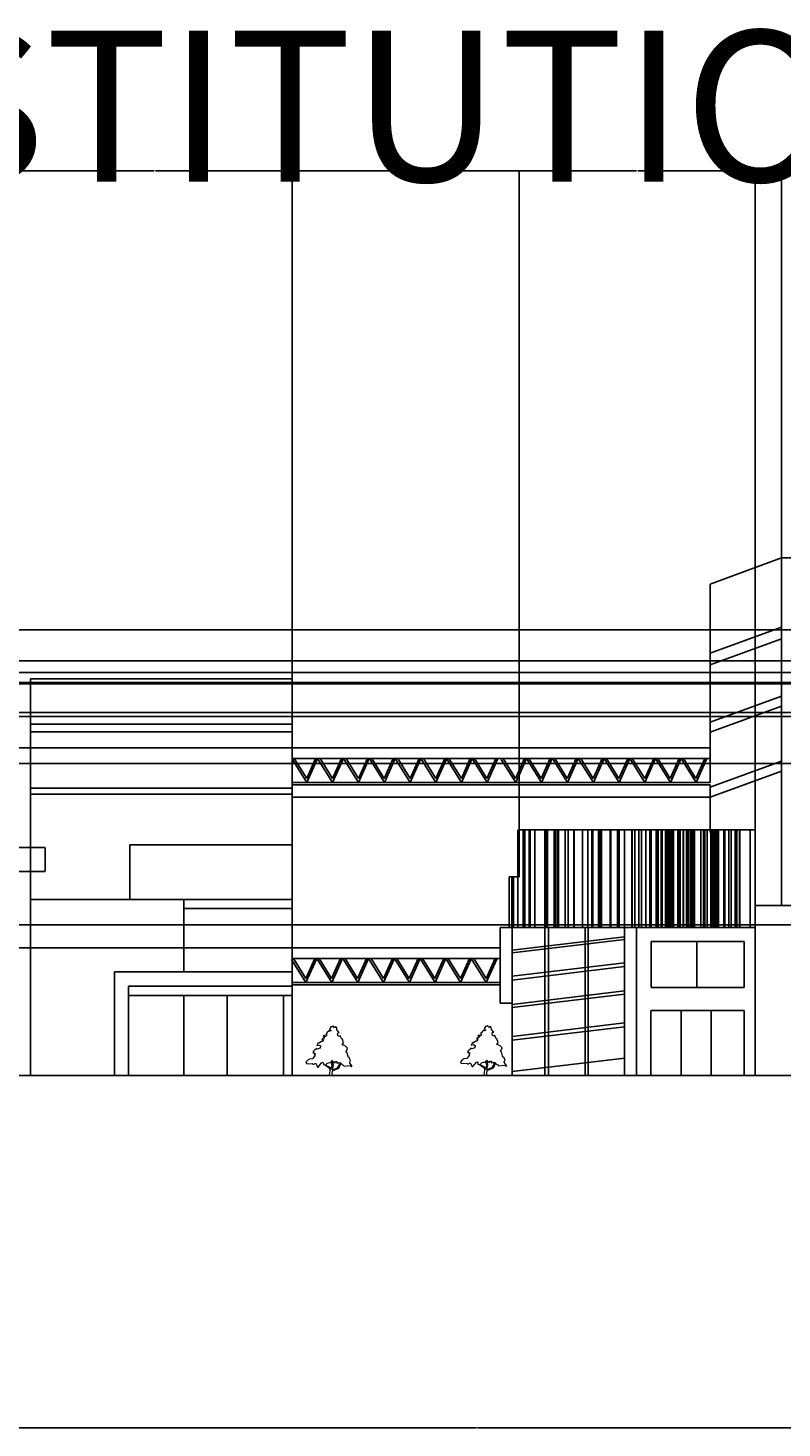
# Model space of a CAD drawing. Units: inches. Extents: x -2248 to 2617, y -128 to 922.
# Tile 4 of 7: x -152 to 413, y -128 to 922. Entities that reach past the tile are written whole.
import ezdxf

# ---------------------------------------------------------------- set-up
doc = ezdxf.new("R2010")
doc.units = ezdxf.units.IN
doc.header["$MEASUREMENT"] = 0
for name, color, linetype, lineweight in [('A-ANNO-DIMS', 2, 'Continuous', 18), ('A-ANNO-TEXT', 7, 'Continuous', 25), ('A-ELEV', 7, 'Continuous', 25), ('L-PLNT', 3, 'Continuous', 18)]:
    doc.layers.add(name, color=color, linetype=linetype, lineweight=lineweight)
doc.styles.get("Standard").update_dxf_attribs({"font": 'arial.ttf'})
doc.dimstyles.get("Standard").update_dxf_attribs({"dimtxt": 0.18, "dimasz": 0.18, "dimexe": 0.18, "dimexo": 0.0625, "dimgap": 0.09, "dimtad": 0, "dimtih": 1, "dimtoh": 1, "dimdec": 4, "dimzin": 0, "dimdsep": 46, "dimtxsty": 'Standard', "dimcen": 0.09, "dimadec": 0, "dimazin": 0, "dimtfac": 1, "dimtdec": 4, "dimtofl": 0, "dimtmove": 0, "dimatfit": 3, "dimfxl": 1, "dimtolj": 1, "dimtzin": 0, "dimarcsym": 0})

# ---------------------------------------------------------------- blocks, each defined once
blk = doc.blocks.new('*U2')
for points in [[(22.0124, 137.721), (18.5475, 141.5624), (15.5282, 138.2446), (13.8028, 139.3505), (13.3714, 142.1153), (11.2148, 143.2214), (8.1954, 140.4564), (4.7447, 141.0094), (2.1567, 136.0326), (2.1567, 131.6088), (5.6074, 129.9499), (3.0193, 128.2909), (0.4313, 130.5029), (-6.9015, 123.3141), (-6.9015, 121.6552), (-9.9208, 119.9963), (-9.0581, 118.3373), (-6.9015, 115.0195), (-10.7835, 112.2546), (-14.6656, 115.0195), (-16.8222, 114.4665), (-17.6849, 112.2546), (-14.6656, 111.7016), (-14.2342, 107.2778), (-17.6065, 107.8307), (-21.5669, 103.9599), (-17.2536, 103.4069), (-18.9789, 97.8771), (-22.8609, 97.3241), (-27.1743, 94.5593), (-32.3504, 91.7944), (-32.7817, 94.0063), (-36.6638, 85.7116), (-29.7624, 87.3705), (-25.449, 84.6056), (-26.743, 77.9699), (-34.507, 75.205), (-37.9578, 77.4169), (-39.2518, 74.099), (-42.2711, 73.5461), (-44.8592, 70.2282), (-47.8786, 66.3574), (-43.9965, 63.0395), (-41.4085, 64.6985), (-44.3346, 59.8898), (-42.2089, 60.1377), (-42.5159, 55.7849), (-49.6039, 46.4502), (-58.2307, 45.8972), (-62.1127, 43.6853), (-68.5828, 36.4966), (-65.9947, 32.0727), (-50.0352, 32.6257), (-47.0159, 30.4138), (-39.6831, 33.7317), (-34.507, 22.6721), (-32.3504, 22.6721), (-22.4296, 34.8376), (-19.4102, 36.4966), (-17.2536, 33.7317), (-17.2536, 29.8608), (-13.8028, 28.7549), (-9.0581, 28.7549), (-7.3328, 32.6257), (-1.7254, 35.3906), (3.8821, 35.9436), (6.4701, 38.1555), (6.9014, 38.7085), (8.1954, 41.4734), (9.9208, 40.3674), (11.2148, 35.9436), (14.2341, 37.6025), (15.0968, 36.4966), (15.9595, 33.7317), (18.9789, 38.7085), (21.9982, 38.7085), (23.2922, 36.4966), (21.9982, 34.2847), (25.4489, 35.3906), (26.743, 33.7317), (29.7623, 35.9436), (32.7817, 34.8376), (38.8204, 28.7549), (41.4084, 27.6489), (43.5651, 25.437), (61.6813, 27.0959), (65.132, 23.7781), (67.7201, 24.884), (60.8186, 33.7317), (60.3873, 37.0495), (62.544, 40.3674), (58.662, 50.874), (56.5053, 50.874), (52.1919, 66.3574), (47.8785, 66.9103), (50.4665, 69.1222), (53.9172, 77.9699), (47.0158, 85.1586), (38.3891, 87.9235), (42.2711, 94.0063)], [(42.2711, 94.0063), (38.8204, 104.5129), (36.6637, 104.5129), (32.3503, 113.9135), (29.7623, 113.3605), (26.743, 113.3605), (24.5862, 117.7844), (25.8802, 123.8671), (29.331, 123.8671), (22.8609, 131.6088), (21.9982, 137.6916)], [(-12.9401, 28.7549), (-2.588, 22.1191), (0.8626, 17.6953), (1.7253, 11.6125), (0, 0)], [(-9.9208, 28.2019), (0, 23.2251), (3.4507, 19.9072), (4.7447, 15.4834), (8.6267, 27.0959), (6.4701, 37.6025)], [(34.5071, 33.1787), (27.1743, 18.2483), (9.0581, 10.5066), (7.7641, 3.8708), (8.1954, 0)], [(8.1954, 40.3674), (11.2148, 27.6489), (8.1954, 13.8245), (24.5862, 19.9072), (32.7817, 34.2847)]]:
    blk.add_lwpolyline(points)
blk = doc.blocks.new('TRUSS-BRIDGE-SEG')
for p, q in [((0, 17.2), (10.8, 0)), ((10.8, 0), (18.9, 17.9)), ((18.8, 17.9), (30.1, 0)), ((30.1, 0), (38.2, 17.9)), ((38.3, 17.9), (49.5, 0)), ((49.5, 0), (57.6, 17.9)), ((57.7, 17.9), (69, 0)), ((69, 0), (77.1, 17.9)), ((77, 17.9), (88.2, 0)), ((88.2, 0), (96.3, 17.9)), ((96.3, 17.9), (107.5, 0)), ((107.5, 0), (115.6, 17.9)), ((115.5, 17.9), (126.7, 0)), ((126.7, 0), (134.8, 17.9)), ((134.7, 17.9), (145.9, 0)), ((145.9, 0), (154, 17.9))]:
    blk.add_line(p, q)
blk = doc.blocks.new('*D15')
at = {"layer": 'A-ANNO-DIMS', "color": 0, "lineweight": -2, "transparency": 16777216}
for p, q in [((-162.3, 307.2), (-139.1, 307.2)), ((-139.3, 307), (-139.3, 298.4)), ((-139.3, 289.5), (-139.3, 298.1)), ((-162.3, 289.3), (-139.1, 289.3))]:
    blk.add_line(p, q, dxfattribs=at)
at = {"layer": 'A-ANNO-DIMS', "color": 0, "transparency": 16777216}
for points in [[(-139.3, 307), (-139.2, 307), (-139.3, 307.2)], [(-139.3, 289.5), (-139.2, 289.5), (-139.3, 289.3)]]:
    blk.add_solid(points, dxfattribs=at)
at = {"layer": 'Defpoints', "color": 0, "transparency": 16777216}
for p in [(-162.4, 307.2), (-139.3, 307.2), (-162.4, 289.3)]:
    blk.add_point(p, dxfattribs=at)
at = {"layer": 'A-ANNO-DIMS', "color": 0, "transparency": 16777216, "insert": (-139.3, 298.2), "char_height": 0.18, "attachment_point": 5}
blk.add_mtext('\\A1;18 TYP.', dxfattribs=at)
blk = doc.blocks.new('*D16')
at = {"layer": 'A-ANNO-DIMS', "color": 0, "lineweight": -2, "transparency": 16777216}
for p, q in [((45.9, 438.4), (2616.5, 438.4)), ((2616.3, 438.3), (2616.3, 287.6)), ((2616.3, 136.6), (2616.3, 287.3)), ((45.9, 136.5), (2616.5, 136.5))]:
    blk.add_line(p, q, dxfattribs=at)
at = {"layer": 'A-ANNO-DIMS', "color": 0, "transparency": 16777216}
for points in [[(2616.2, 438.3), (2616.3, 438.3), (2616.3, 438.4)], [(2616.2, 136.6), (2616.3, 136.6), (2616.3, 136.5)]]:
    blk.add_solid(points, dxfattribs=at)
at = {"layer": 'Defpoints', "color": 0, "transparency": 16777216}
for p in [(45.8, 438.4), (45.8, 136.5), (2616.3, 136.5)]:
    blk.add_point(p, dxfattribs=at)
at = {"layer": 'A-ANNO-DIMS', "color": 0, "transparency": 16777216, "insert": (2616.3, 287.4), "char_height": 0.18, "attachment_point": 5}
blk.add_mtext('\\A1;302', dxfattribs=at)
blk = doc.blocks.new('*D20')
at = {"layer": 'A-ANNO-DIMS', "color": 0, "lineweight": -2, "transparency": 16777216}
for p, q in [((-1595.3, 429.9), (2616.5, 429.9)), ((2616.3, 429.7), (2616.3, 417.9)), ((2616.3, 405.8), (2616.3, 417.5)), ((-1653.9, 405.6), (2616.5, 405.6))]:
    blk.add_line(p, q, dxfattribs=at)
at = {"layer": 'A-ANNO-DIMS', "color": 0, "transparency": 16777216}
for points in [[(2616.2, 429.7), (2616.3, 429.7), (2616.3, 429.9)], [(2616.2, 405.8), (2616.3, 405.8), (2616.3, 405.6)]]:
    blk.add_solid(points, dxfattribs=at)
at = {"layer": 'Defpoints', "color": 0, "transparency": 16777216}
for p in [(-1595.4, 429.9), (-1654, 405.6), (2616.3, 405.6)]:
    blk.add_point(p, dxfattribs=at)
at = {"layer": 'A-ANNO-DIMS', "color": 0, "transparency": 16777216, "insert": (2616.3, 417.7), "char_height": 0.18, "attachment_point": 5}
blk.add_mtext('\\A1;24.3', dxfattribs=at)
blk = doc.blocks.new('*D21')
at = {"layer": 'A-ANNO-DIMS', "color": 0, "lineweight": -2, "transparency": 16777216}
for p, q in [((-1125.3, 470.6), (2616.5, 470.6)), ((2616.3, 470.4), (2616.3, 451)), ((2616.3, 431.1), (2616.3, 450.6)), ((-1257.9, 430.9), (2616.5, 430.9))]:
    blk.add_line(p, q, dxfattribs=at)
at = {"layer": 'A-ANNO-DIMS', "color": 0, "transparency": 16777216}
for points in [[(2616.2, 470.4), (2616.3, 470.4), (2616.3, 470.6)], [(2616.2, 431.1), (2616.3, 431.1), (2616.3, 430.9)]]:
    blk.add_solid(points, dxfattribs=at)
at = {"layer": 'Defpoints', "color": 0, "transparency": 16777216}
for p in [(-1125.4, 470.6), (-1258, 430.9), (2616.3, 430.9)]:
    blk.add_point(p, dxfattribs=at)
at = {"layer": 'A-ANNO-DIMS', "color": 0, "transparency": 16777216, "insert": (2616.3, 450.8), "char_height": 0.18, "attachment_point": 5}
blk.add_mtext('\\A1;39.705', dxfattribs=at)
blk = doc.blocks.new('*D22')
at = {"layer": 'A-ANNO-DIMS', "color": 0, "lineweight": -2, "transparency": 16777216}
for p, q in [((-733.3, 408.4), (2616.5, 408.4)), ((2616.3, 408.2), (2616.3, 329.1)), ((2616.3, 249.6), (2616.3, 328.7)), ((-719.1, 249.4), (2616.5, 249.4))]:
    blk.add_line(p, q, dxfattribs=at)
at = {"layer": 'A-ANNO-DIMS', "color": 0, "transparency": 16777216}
for points in [[(2616.2, 408.2), (2616.3, 408.2), (2616.3, 408.4)], [(2616.2, 249.6), (2616.3, 249.6), (2616.3, 249.4)]]:
    blk.add_solid(points, dxfattribs=at)
at = {"layer": 'Defpoints', "color": 0, "transparency": 16777216}
for p in [(-733.4, 408.4), (-719.2, 249.4), (2616.3, 249.4)]:
    blk.add_point(p, dxfattribs=at)
at = {"layer": 'A-ANNO-DIMS', "color": 0, "transparency": 16777216, "insert": (2616.3, 328.9), "char_height": 0.18, "attachment_point": 5}
blk.add_mtext('\\A1;159.02', dxfattribs=at)
blk = doc.blocks.new('*D23')
at = {"layer": 'A-ANNO-DIMS', "color": 0, "lineweight": -2, "transparency": 16777216}
for p, q in [((-719.1, 249.4), (2616.5, 249.4)), ((2616.3, 249.2), (2616.3, 193.1)), ((2616.3, 136.6), (2616.3, 192.7)), ((-719.1, 136.5), (2616.5, 136.5))]:
    blk.add_line(p, q, dxfattribs=at)
at = {"layer": 'A-ANNO-DIMS', "color": 0, "transparency": 16777216}
for points in [[(2616.2, 249.2), (2616.3, 249.2), (2616.3, 249.4)], [(2616.2, 136.6), (2616.3, 136.6), (2616.3, 136.5)]]:
    blk.add_solid(points, dxfattribs=at)
at = {"layer": 'Defpoints', "color": 0, "transparency": 16777216}
for p in [(-719.2, 249.4), (-719.2, 136.5), (2616.3, 136.5)]:
    blk.add_point(p, dxfattribs=at)
at = {"layer": 'A-ANNO-DIMS', "color": 0, "transparency": 16777216, "insert": (2616.3, 192.9), "char_height": 0.18, "attachment_point": 5}
blk.add_mtext('\\A1;112.94', dxfattribs=at)
blk = doc.blocks.new('*D24')
at = {"layer": 'A-ANNO-DIMS', "color": 0, "lineweight": -2, "transparency": 16777216}
for p, q in [((-316.1, 370.3), (2616.5, 370.3)), ((2616.3, 370.1), (2616.3, 253.6)), ((2616.3, 136.6), (2616.3, 253.2)), ((-159.8, 136.5), (2616.5, 136.5))]:
    blk.add_line(p, q, dxfattribs=at)
at = {"layer": 'A-ANNO-DIMS', "color": 0, "transparency": 16777216}
for points in [[(2616.2, 370.1), (2616.3, 370.1), (2616.3, 370.3)], [(2616.2, 136.6), (2616.3, 136.6), (2616.3, 136.5)]]:
    blk.add_solid(points, dxfattribs=at)
at = {"layer": 'Defpoints', "color": 0, "transparency": 16777216}
for p in [(-316.2, 370.3), (-159.9, 136.5), (2616.3, 136.5)]:
    blk.add_point(p, dxfattribs=at)
at = {"layer": 'A-ANNO-DIMS', "color": 0, "transparency": 16777216, "insert": (2616.3, 253.4), "char_height": 0.18, "attachment_point": 5}
blk.add_mtext('\\A1;233.87', dxfattribs=at)
blk = doc.blocks.new('*D29')
at = {"layer": 'A-ANNO-DIMS', "color": 0, "lineweight": -2, "transparency": 16777216}
for p, q in [((358.9, 382), (-2247.7, 382)), ((-2247.5, 381.8), (-2247.5, 259.4)), ((-2247.5, 136.6), (-2247.5, 259)), ((392.6, 136.5), (-2247.7, 136.5))]:
    blk.add_line(p, q, dxfattribs=at)
at = {"layer": 'A-ANNO-DIMS', "color": 0, "transparency": 16777216}
for points in [[(-2247.5, 381.8), (-2247.5, 381.8), (-2247.5, 382)], [(-2247.5, 136.6), (-2247.5, 136.6), (-2247.5, 136.5)]]:
    blk.add_solid(points, dxfattribs=at)
at = {"layer": 'Defpoints', "color": 0, "transparency": 16777216}
for p in [(359, 382), (-2247.5, 136.5), (392.7, 136.5)]:
    blk.add_point(p, dxfattribs=at)
at = {"layer": 'A-ANNO-DIMS', "color": 0, "transparency": 16777216, "insert": (-2247.5, 259.2), "char_height": 0.18, "attachment_point": 5}
blk.add_mtext('\\A1;245.5', dxfattribs=at)
blk = doc.blocks.new('*D30')
at = {"layer": 'A-ANNO-DIMS', "color": 0, "lineweight": -2, "transparency": 16777216}
for p, q in [((201.8, 232.1), (-2247.7, 232.1)), ((-2247.5, 231.9), (-2247.5, 184.4)), ((-2247.5, 136.6), (-2247.5, 184.1)), ((210.7, 136.5), (-2247.7, 136.5))]:
    blk.add_line(p, q, dxfattribs=at)
at = {"layer": 'A-ANNO-DIMS', "color": 0, "transparency": 16777216}
for points in [[(-2247.5, 231.9), (-2247.5, 231.9), (-2247.5, 232.1)], [(-2247.5, 136.6), (-2247.5, 136.6), (-2247.5, 136.5)]]:
    blk.add_solid(points, dxfattribs=at)
at = {"layer": 'Defpoints', "color": 0, "transparency": 16777216}
for p in [(201.8, 232.1), (-2247.5, 136.5), (210.8, 136.5)]:
    blk.add_point(p, dxfattribs=at)
at = {"layer": 'A-ANNO-DIMS', "color": 0, "transparency": 16777216, "insert": (-2247.5, 184.3), "char_height": 0.18, "attachment_point": 5}
blk.add_mtext('\\A1;95.6', dxfattribs=at)
blk = doc.blocks.new('*D31')
at = {"layer": 'A-ANNO-DIMS', "color": 0, "lineweight": -2, "transparency": 16777216}
for p, q in [((934.8, 447.2), (-2247.7, 447.2)), ((-2247.5, 447), (-2247.5, 292)), ((-2247.5, 136.6), (-2247.5, 291.6)), ((820, 136.5), (-2247.7, 136.5))]:
    blk.add_line(p, q, dxfattribs=at)
at = {"layer": 'A-ANNO-DIMS', "color": 0, "transparency": 16777216}
for points in [[(-2247.5, 447), (-2247.5, 447), (-2247.5, 447.2)], [(-2247.5, 136.6), (-2247.5, 136.6), (-2247.5, 136.5)]]:
    blk.add_solid(points, dxfattribs=at)
at = {"layer": 'Defpoints', "color": 0, "transparency": 16777216}
for p in [(934.9, 447.2), (-2247.5, 136.5), (820.1, 136.5)]:
    blk.add_point(p, dxfattribs=at)
at = {"layer": 'A-ANNO-DIMS', "color": 0, "transparency": 16777216, "insert": (-2247.5, 291.8), "char_height": 0.18, "attachment_point": 5}
blk.add_mtext('\\A1;310.7', dxfattribs=at)
blk = doc.blocks.new('*D33')
at = {"layer": 'A-ANNO-DIMS', "color": 0, "lineweight": -2, "transparency": 16777216}
for p, q in [((2393, 136.4), (2393, -127.9)), ((-2024.3, 122), (-2024.3, -127.9)), ((-2024.1, -127.7), (184, -127.7)), ((2392.8, -127.7), (184.7, -127.7))]:
    blk.add_line(p, q, dxfattribs=at)
at = {"layer": 'A-ANNO-DIMS', "color": 0, "transparency": 16777216}
for points in [[(-2024.1, -127.6), (-2024.1, -127.7), (-2024.3, -127.7)], [(2392.8, -127.6), (2392.8, -127.7), (2393, -127.7)]]:
    blk.add_solid(points, dxfattribs=at)
at = {"layer": 'Defpoints', "color": 0, "transparency": 16777216}
for p in [(2393, 136.5), (-2024.3, 122.1), (2393, -127.7)]:
    blk.add_point(p, dxfattribs=at)
at = {"layer": 'A-ANNO-DIMS', "color": 0, "transparency": 16777216, "insert": (184.4, -127.7), "char_height": 0.18, "attachment_point": 5}
blk.add_mtext('\\A1;4417', dxfattribs=at)
blk = doc.blocks.new('*D45')
at = {"layer": 'A-ANNO-DIMS', "color": 0, "lineweight": -2, "transparency": 16777216}
for p, q in [((-159.9, 438.5), (-159.9, 814.7)), ((-159.7, 814.5), (-57.5, 814.5)), ((45.6, 814.5), (-56.6, 814.5)), ((45.8, 438.5), (45.8, 814.7))]:
    blk.add_line(p, q, dxfattribs=at)
at = {"layer": 'A-ANNO-DIMS', "color": 0, "transparency": 16777216}
for points in [[(-159.7, 814.5), (-159.7, 814.5), (-159.9, 814.5)], [(45.6, 814.5), (45.6, 814.5), (45.8, 814.5)]]:
    blk.add_solid(points, dxfattribs=at)
at = {"layer": 'Defpoints', "color": 0, "transparency": 16777216}
for p in [(45.8, 814.5), (-159.9, 438.4), (45.8, 438.4)]:
    blk.add_point(p, dxfattribs=at)
at = {"layer": 'A-ANNO-DIMS', "color": 0, "transparency": 16777216, "insert": (-57, 814.5), "char_height": 0.18, "attachment_point": 5}
blk.add_mtext('\\A1;205.73', dxfattribs=at)
blk = doc.blocks.new('*D46')
at = {"layer": 'A-ANNO-DIMS', "color": 0, "lineweight": -2, "transparency": 16777216}
for p, q in [((45.8, 438.5), (45.8, 814.7)), ((46, 814.5), (130.5, 814.5)), ((215.8, 814.5), (131.2, 814.5)), ((215.9, 320.7), (215.9, 814.7))]:
    blk.add_line(p, q, dxfattribs=at)
at = {"layer": 'A-ANNO-DIMS', "color": 0, "transparency": 16777216}
for points in [[(46, 814.5), (46, 814.5), (45.8, 814.5)], [(215.8, 814.5), (215.8, 814.5), (215.9, 814.5)]]:
    blk.add_solid(points, dxfattribs=at)
at = {"layer": 'Defpoints', "color": 0, "transparency": 16777216}
for p in [(215.9, 814.5), (45.8, 438.4), (215.9, 320.6)]:
    blk.add_point(p, dxfattribs=at)
at = {"layer": 'A-ANNO-DIMS', "color": 0, "transparency": 16777216, "insert": (130.9, 814.5), "char_height": 0.18, "attachment_point": 5}
blk.add_mtext('\\A1;170.1', dxfattribs=at)
blk = doc.blocks.new('*D47')
at = {"layer": 'A-ANNO-DIMS', "color": 0, "lineweight": -2, "transparency": 16777216}
for p, q in [((215.9, 320.7), (215.9, 814.7)), ((216.1, 814.5), (303.9, 814.5)), ((392.5, 814.5), (304.8, 814.5)), ((392.7, 320.7), (392.7, 814.7))]:
    blk.add_line(p, q, dxfattribs=at)
at = {"layer": 'A-ANNO-DIMS', "color": 0, "transparency": 16777216}
for points in [[(216.1, 814.5), (216.1, 814.5), (215.9, 814.5)], [(392.5, 814.5), (392.5, 814.5), (392.7, 814.5)]]:
    blk.add_solid(points, dxfattribs=at)
at = {"layer": 'Defpoints', "color": 0, "transparency": 16777216}
for p in [(392.7, 814.5), (215.9, 320.6), (392.7, 320.6)]:
    blk.add_point(p, dxfattribs=at)
at = {"layer": 'A-ANNO-DIMS', "color": 0, "transparency": 16777216, "insert": (304.3, 814.5), "char_height": 0.18, "attachment_point": 5}
blk.add_mtext('\\A1;176.76', dxfattribs=at)
blk = doc.blocks.new('*D48')
at = {"layer": 'A-ANNO-DIMS', "color": 0, "lineweight": -2, "transparency": 16777216}
for p, q in [((392.7, 320.7), (392.7, 814.7)), ((392.9, 814.5), (402.2, 814.5)), ((412.4, 814.5), (403.1, 814.5)), ((412.6, 524.4), (412.6, 814.7))]:
    blk.add_line(p, q, dxfattribs=at)
at = {"layer": 'A-ANNO-DIMS', "color": 0, "transparency": 16777216}
for points in [[(392.9, 814.5), (392.9, 814.5), (392.7, 814.5)], [(412.4, 814.5), (412.4, 814.5), (412.6, 814.5)]]:
    blk.add_solid(points, dxfattribs=at)
at = {"layer": 'Defpoints', "color": 0, "transparency": 16777216}
for p in [(412.6, 814.5), (412.6, 524.3), (392.7, 320.6)]:
    blk.add_point(p, dxfattribs=at)
at = {"layer": 'A-ANNO-DIMS', "color": 0, "transparency": 16777216, "insert": (402.7, 814.5), "char_height": 0.18, "attachment_point": 5}
blk.add_mtext('\\A1;19.923', dxfattribs=at)
blk = doc.blocks.new('*D49')
at = {"layer": 'A-ANNO-DIMS', "color": 0, "lineweight": -2, "transparency": 16777216}
for p, q in [((412.6, 524.4), (412.6, 814.7)), ((412.8, 814.5), (518.4, 814.5)), ((624.9, 814.5), (519.3, 814.5)), ((625.1, 524.4), (625.1, 814.7))]:
    blk.add_line(p, q, dxfattribs=at)
at = {"layer": 'A-ANNO-DIMS', "color": 0, "transparency": 16777216}
for points in [[(412.8, 814.5), (412.8, 814.5), (412.6, 814.5)], [(624.9, 814.5), (624.9, 814.5), (625.1, 814.5)]]:
    blk.add_solid(points, dxfattribs=at)
at = {"layer": 'Defpoints', "color": 0, "transparency": 16777216}
for p in [(625.1, 814.5), (412.6, 524.3), (625.1, 524.3)]:
    blk.add_point(p, dxfattribs=at)
at = {"layer": 'A-ANNO-DIMS', "color": 0, "transparency": 16777216, "insert": (518.8, 814.5), "char_height": 0.18, "attachment_point": 5}
blk.add_mtext('\\A1;212.44', dxfattribs=at)

msp = doc.modelspace()

# ---------------------------------------------------------------- linework, layer by layer
at = {"layer": 'A-ELEV'}
for p, q in [((358.982, 504.797), (412.6205, 524.3284)), ((412.6205, 524.3284), (412.6205, 263.9212)), ((412.6205, 524.3284), (625.0568, 524.3284)), ((358.982, 381.9653), (358.982, 504.797)), ((358.982, 453.0174), (412.6205, 472.5488)), ((358.982, 444.141), (412.6205, 463.6724)), ((-159.9067, 438.443), (3.2456, 438.443)), ((-150.228, 136.4519), (-150.228, 433.7073)), ((-150.228, 433.7073), (45.827, 433.7073)), ((3.2456, 438.443), (45.827, 438.443)), ((45.827, 438.443), (45.827, 136.4519)), ((358.982, 401.2379), (412.6205, 420.7693)), ((358.982, 393.8408), (412.6205, 413.3722)), ((-150.228, 399.7951), (45.827, 399.7951)), ((-150.228, 393.8999), (45.827, 393.8999)), ((93.8585, 381.9653), (46.0493, 381.9653)), ((93.8585, 381.9653), (202.4585, 381.9653)), ((198.9373, 381.9653), (202.4585, 381.9653)), ((250.382, 381.9653), (202.5728, 381.9653)), ((250.382, 381.9653), (358.982, 381.9653)), ((355.4608, 381.9653), (358.982, 381.9653)), ((358.982, 357.5233), (358.982, 381.9653)), ((46.0493, 373.9955), (202.4585, 373.9955)), ((47.4623, 373.9898), (56.7416, 359.1374)), ((56.7416, 359.1374), (63.4542, 373.9955)), ((66.7389, 373.9898), (76.0183, 359.1374)), ((76.0183, 359.1374), (82.7309, 373.9955)), ((86.2159, 373.9898), (95.4952, 359.1374)), ((95.4952, 359.1374), (102.2078, 373.9955)), ((105.6355, 373.9898), (114.9149, 359.1374)), ((114.9149, 359.1374), (121.6275, 373.9955)), ((124.9224, 373.9898), (134.2018, 359.1374)), ((134.2018, 359.1374), (140.9144, 373.9955)), ((144.2094, 373.9898), (153.4887, 359.1374)), ((153.4887, 359.1374), (160.2013, 373.9955)), ((163.349, 373.9898), (172.6283, 359.1374)), ((172.6283, 359.1374), (179.3409, 373.9955)), ((182.5409, 373.9898), (191.8203, 359.1374)), ((191.8203, 359.1374), (198.5328, 373.9955)), ((202.5728, 373.9955), (358.982, 373.9955)), ((203.9858, 373.9898), (213.2651, 359.1374)), ((213.2651, 359.1374), (219.9777, 373.9955)), ((223.2624, 373.9898), (232.5418, 359.1374)), ((232.5418, 359.1374), (239.2544, 373.9955)), ((242.7394, 373.9898), (252.0187, 359.1374)), ((252.0187, 359.1374), (258.7313, 373.9955)), ((262.159, 373.9898), (271.4384, 359.1374)), ((271.4384, 359.1374), (278.151, 373.9955)), ((281.4459, 373.9898), (290.7253, 359.1374)), ((290.7253, 359.1374), (297.4379, 373.9955)), ((300.7329, 373.9898), (310.0122, 359.1374)), ((310.0122, 359.1374), (316.7248, 373.9955)), ((319.8725, 373.9898), (329.1518, 359.1374)), ((329.1518, 359.1374), (335.8644, 373.9955)), ((339.0644, 373.9898), (348.3438, 359.1374)), ((348.3438, 359.1374), (355.0563, 373.9955)), ((358.982, 352.4172), (412.6205, 371.9486)), ((358.982, 345.0201), (412.6205, 364.5515)), ((358.982, 357.5233), (358.982, 356.0447)), ((-150.228, 351.7702), (45.827, 351.7702)), ((-150.228, 347.2778), (45.827, 347.2778)), ((46.0493, 356.0447), (194.121, 356.0447)), ((55.3542, 354.2906), (46.0493, 354.2906)), ((55.3542, 354.2906), (182.3725, 354.2906)), ((151.1439, 356.0447), (151.1588, 356.0121)), ((151.1588, 356.0121), (151.1767, 356.0447)), ((182.3725, 354.2906), (194.121, 354.2906)), ((194.121, 356.0447), (195.7759, 356.0447)), ((194.121, 354.2906), (202.4585, 354.2906)), ((202.4585, 356.0447), (195.7759, 356.0447)), ((202.5728, 356.0447), (350.6445, 356.0447)), ((211.8777, 354.2906), (202.5728, 354.2906)), ((211.8777, 354.2906), (338.896, 354.2906)), ((307.6674, 356.0447), (307.6823, 356.0121)), ((307.6823, 356.0121), (307.7002, 356.0447)), ((338.896, 354.2906), (350.6445, 354.2906)), ((350.6445, 356.0447), (352.2994, 356.0447)), ((350.6445, 354.2906), (358.982, 354.2906)), ((358.982, 356.0447), (352.2994, 356.0447)), ((358.982, 354.2906), (358.982, 345.0201)), ((358.982, 345.0201), (45.827, 345.0201)), ((358.982, 345.0201), (358.982, 318.6086)), ((214.9376, 320.6034), (214.9376, 247.4133)), ((215.9358, 285.4051), (215.9358, 320.6034)), ((215.9358, 320.6034), (392.6975, 320.6034)), ((219.0022, 320.6034), (219.0022, 247.4133)), ((220.1107, 320.6034), (220.1107, 247.4133)), ((223.4363, 320.6034), (223.4363, 247.4133)), ((224.1753, 320.6034), (224.1753, 247.4133)), ((227.6322, 320.6034), (227.6322, 247.4133)), ((235.2347, 320.6034), (235.2347, 247.4133)), ((235.9997, 320.6034), (235.9997, 247.4133)), ((237.1082, 320.6034), (237.1082, 247.4133)), ((242.2814, 320.6034), (242.2814, 247.4133)), ((242.8371, 320.6034), (242.8371, 247.4133)), ((244.4129, 320.6034), (244.4129, 247.4133)), ((245.2375, 320.6034), (245.2375, 247.4133)), ((245.3368, 320.6034), (245.3368, 247.4133)), ((250.4395, 320.6034), (250.4395, 247.4133)), ((252.6277, 320.6034), (252.6277, 247.4133)), ((256.9559, 320.6034), (256.9559, 247.4133)), ((257.0618, 320.6034), (257.0618, 247.4133)), ((263.4723, 320.6034), (263.4723, 247.4133)), ((267.2785, 320.6034), (267.2785, 247.4133)), ((270.5121, 320.6034), (270.5121, 247.4133)), ((270.974, 320.6034), (270.974, 247.4133)), ((271.0747, 320.6034), (271.0747, 247.4133)), ((271.205, 320.6034), (271.205, 247.4133)), ((275.3624, 320.6034), (275.3624, 247.4133)), ((276.6459, 320.6034), (276.6459, 247.4133)), ((277.591, 320.6034), (277.591, 247.4133)), ((284.1074, 320.6034), (284.1074, 247.4133)), ((284.139, 320.6034), (284.139, 247.4133)), ((284.601, 320.6034), (284.601, 247.4133)), ((289.5377, 320.6034), (289.5377, 247.4133)), ((289.9132, 320.6034), (289.9132, 247.4133)), ((290.8371, 320.6034), (290.8371, 247.4133)), ((294.968, 320.6034), (294.968, 247.4133)), ((294.968, 320.6034), (294.968, 252.6663)), ((294.968, 320.6034), (294.968, 251.7436)), ((294.968, 320.6034), (294.968, 265.9324)), ((294.968, 317.0902), (294.968, 243.9001)), ((300.3067, 320.6034), (300.3067, 247.4133)), ((300.6642, 320.6034), (300.6642, 247.4133)), ((302.5117, 320.6034), (302.5117, 247.4133)), ((305.6189, 320.6034), (305.6189, 247.4133)), ((307.6976, 320.6034), (307.6976, 247.4133)), ((310.9311, 320.6034), (310.9311, 247.4133)), ((310.9311, 320.6034), (310.9311, 247.4133)), ((313.9337, 320.6034), (313.9337, 247.4133)), ((313.9337, 320.6034), (313.9337, 247.4133)), ((314.8575, 320.6034), (314.8575, 247.4133)), ((318.553, 320.6034), (318.553, 247.4133)), ((318.7839, 320.6034), (318.7839, 247.4133)), ((318.7839, 320.6034), (318.7839, 247.4133)), ((319.7078, 320.6034), (319.7078, 247.4133)), ((320.1697, 320.6034), (320.1697, 247.4133)), ((322.2484, 320.6034), (322.2484, 247.4133)), ((323.1723, 320.6034), (323.1723, 247.4133)), ((325.482, 320.6034), (325.482, 247.4133)), ((325.9439, 320.6034), (325.9439, 247.4133)), ((326.5299, 320.6034), (326.5299, 247.4133)), ((327.3297, 320.6034), (327.3297, 247.4133)), ((328.0226, 320.6034), (328.0226, 247.4133)), ((328.4845, 320.6034), (328.4845, 247.4133)), ((328.7155, 320.6034), (328.7155, 247.4133)), ((329.6393, 320.6034), (329.6393, 247.4133)), ((330.3322, 320.6034), (330.3322, 247.4133)), ((331.4871, 320.6034), (331.4871, 247.4133)), ((331.4871, 320.6034), (331.4871, 247.4133)), ((334.7206, 320.6034), (334.7206, 247.4133)), ((335.4135, 320.6034), (335.4135, 247.4133)), ((336.3374, 320.6034), (336.3374, 247.4133)), ((336.5683, 320.6034), (336.5683, 247.4133)), ((338.878, 320.6034), (338.878, 247.4133)), ((339.1089, 320.6034), (339.1089, 247.4133)), ((341.4186, 320.6034), (341.4186, 247.4133)), ((342.1115, 320.6034), (342.1115, 247.4133)), ((342.5734, 320.6034), (342.5734, 247.4133)), ((343.9592, 320.6034), (343.9592, 247.4133)), ((344.8831, 320.6034), (344.8831, 247.4133)), ((345.576, 320.6034), (345.576, 247.4133)), ((346.2689, 320.6034), (346.2689, 247.4133)), ((346.9618, 320.6034), (346.9618, 247.4133)), ((347.1927, 320.6034), (347.1927, 247.4133)), ((347.4237, 320.6034), (347.4237, 247.4133)), ((347.4237, 320.6034), (347.4237, 247.4133)), ((352.043, 320.6034), (352.043, 247.4133)), ((354.1217, 320.6034), (354.1217, 247.4133)), ((355.0456, 320.6034), (355.0456, 247.4133)), ((356.8933, 320.6034), (356.8933, 247.4133)), ((359.6649, 320.6034), (359.6649, 247.4133)), ((360.3578, 320.6034), (360.3578, 247.4133)), ((361.0507, 320.6034), (361.0507, 247.4133)), ((361.5126, 320.6034), (361.5126, 247.4133)), ((362.6675, 320.6034), (362.6675, 247.4133)), ((362.8984, 320.6034), (362.8984, 247.4133)), ((363.5913, 320.6034), (363.5913, 247.4133)), ((364.2842, 320.6034), (364.2842, 247.4133)), ((365.2081, 320.6034), (365.2081, 247.4133)), ((369.3655, 320.6034), (369.3655, 247.4133)), ((370.0584, 320.6034), (370.0584, 247.4133)), ((373.0609, 320.6034), (373.0609, 247.4133)), ((374.6777, 320.6034), (374.6777, 247.4133)), ((377.9112, 320.6034), (377.9112, 247.4133)), ((379.066, 320.6034), (379.066, 247.4133)), ((380.9138, 320.6034), (380.9138, 247.4133)), ((381.3757, 320.6034), (381.3757, 247.4133)), ((388.9976, 320.6034), (388.9976, 247.4133)), ((392.6975, 320.6034), (392.6975, 247.4133)), ((-75.8454, 268.3497), (-75.8454, 309.1893)), ((-75.8454, 309.1893), (45.827, 309.1893)), ((208.5456, 247.4133), (208.5456, 285.4051)), ((208.5456, 285.4051), (215.9358, 285.4051)), ((210.5034, 285.4051), (210.5034, 247.4133)), ((211.612, 285.4051), (211.612, 247.4133)), ((-150.228, 268.3497), (45.827, 268.3497)), ((-35.4162, 267.6905), (-35.4162, 268.3497)), ((-35.4162, 214.0412), (-35.4162, 267.6905)), ((412.6205, 263.9212), (392.6975, 263.9212)), ((455.0751, 263.9212), (412.6205, 263.9212)), ((-35.4162, 261.6361), (45.827, 261.6361)), ((208.5456, 247.4133), (201.8252, 247.4133)), ((201.8252, 247.4133), (201.8252, 190.6132)), ((392.6975, 247.4133), (208.5456, 247.4133)), ((210.7789, 247.4133), (210.7789, 136.4519)), ((235.2347, 247.4133), (235.2347, 136.4519)), ((237.8514, 247.4133), (237.8514, 136.4519)), ((265.3272, 247.4133), (265.3272, 136.4519)), ((267.595, 247.4133), (267.595, 136.4519)), ((294.968, 247.4133), (294.968, 136.4519)), ((303.7739, 247.4133), (303.7739, 136.4519)), ((392.6975, 247.4133), (392.6975, 136.4519)), ((93.2252, 232.0521), (45.416, 232.0521)), ((93.2252, 232.0521), (201.8252, 232.0521)), ((198.304, 232.0521), (201.8252, 232.0521)), ((201.8252, 207.61), (201.8252, 232.0521)), ((210.7789, 230.238), (294.968, 240.3368)), ((210.7789, 228.2782), (294.968, 238.3771)), ((384.5194, 236.7167), (314.7736, 236.7167)), ((314.7736, 236.7167), (314.7736, 230.1859)), ((349.1016, 236.7167), (349.1016, 202.4298)), ((384.5194, 202.4298), (384.5194, 236.7167)), ((45.416, 224.0823), (201.8252, 224.0823)), ((45.416, 223.3988), (56.193, 206.1492)), ((46.8289, 224.0766), (56.1083, 209.2241)), ((56.1083, 209.2241), (62.8209, 224.0823)), ((56.193, 206.1492), (64.2941, 224.0809)), ((64.2656, 224.0823), (75.4696, 206.1492)), ((66.1056, 224.0766), (75.385, 209.2241)), ((75.385, 209.2241), (82.0975, 224.0823)), ((75.4696, 206.1492), (83.5708, 224.0809)), ((83.7426, 224.0823), (94.9466, 206.1492)), ((85.5825, 224.0766), (94.8619, 209.2241)), ((94.8619, 209.2241), (101.5745, 224.0823)), ((94.9466, 206.1492), (103.0477, 224.0809)), ((103.1622, 224.0823), (114.3662, 206.1492)), ((105.0022, 224.0766), (114.2815, 209.2241)), ((114.2815, 209.2241), (120.9941, 224.0823)), ((114.3662, 206.1492), (122.4674, 224.0809)), ((122.4491, 224.0823), (133.6532, 206.1492)), ((124.2891, 224.0766), (133.5685, 209.2241)), ((133.5685, 209.2241), (140.2811, 224.0823)), ((133.6532, 206.1492), (141.7543, 224.0809)), ((141.7361, 224.0823), (152.9401, 206.1492)), ((143.576, 224.0766), (152.8554, 209.2241)), ((152.8554, 209.2241), (159.568, 224.0823)), ((152.9401, 206.1492), (161.0412, 224.0809)), ((160.8757, 224.0823), (172.0797, 206.1492)), ((162.7157, 224.0766), (171.995, 209.2241)), ((171.995, 209.2241), (178.7076, 224.0823)), ((172.0797, 206.1492), (180.1808, 224.0809)), ((180.0676, 224.0823), (191.2716, 206.1492)), ((181.9076, 224.0766), (191.1869, 209.2241)), ((191.1869, 209.2241), (197.8995, 224.0823)), ((191.2716, 206.1492), (199.3727, 224.0809)), ((210.7789, 210.806), (294.968, 220.9048)), ((314.7736, 230.1859), (314.7736, 202.4298)), ((-87.3742, 136.4519), (-87.3742, 214.0412)), ((-87.3742, 214.0412), (45.827, 214.0412)), ((210.7789, 207.9753), (294.968, 218.0741)), ((-76.7236, 136.4519), (-76.7236, 203.4034)), ((-76.7236, 203.4034), (45.827, 203.4034)), ((45.416, 206.1315), (193.4877, 206.1315)), ((54.7209, 204.3774), (45.416, 204.3774)), ((54.7209, 204.3774), (181.7392, 204.3774)), ((150.5106, 206.1315), (150.5255, 206.0988)), ((150.5255, 206.0988), (150.5434, 206.1315)), ((181.7392, 204.3774), (193.4877, 204.3774)), ((193.4877, 206.1315), (195.1426, 206.1315)), ((193.4877, 204.3774), (201.8252, 204.3774)), ((201.8252, 206.1315), (195.1426, 206.1315)), ((201.8252, 207.61), (201.8252, 206.1315)), ((210.7789, 189.6431), (294.968, 199.7419)), ((314.7736, 202.4298), (384.5194, 202.4298)), ((-76.7236, 196.3079), (45.827, 196.3079)), ((-35.4162, 196.3079), (-35.4162, 136.4519)), ((-2.8259, 196.3079), (-2.8259, 136.4519)), ((39.4522, 196.3079), (39.4522, 136.4519)), ((201.8252, 190.6132), (210.7789, 190.6132)), ((210.7789, 187.2478), (294.968, 197.3467)), ((314.5301, 185.0391), (314.5301, 136.4519)), ((314.7736, 185.0391), (384.5194, 185.0391)), ((337.4048, 185.0391), (337.4048, 136.4519)), ((359.8479, 185.0391), (359.8479, 136.4519)), ((384.5194, 185.0391), (384.5194, 136.4519)), ((210.7789, 165.6726), (294.968, 175.7715)), ((210.7789, 162.8601), (294.968, 172.9589)), ((210.7789, 139.2727), (294.968, 149.3716)), ((-602.3282, 136.4519), (517.5185, 136.4519))]:
    msp.add_line(p, q, dxfattribs=at)

# ---------------------------------------------------------------- block references
for p in [(46.0492, 356.0623), (202.5727, 356.0623)]:
    msp.add_blockref('TRUSS-BRIDGE-SEG', p, dxfattribs=at)
at = {"layer": 'L-PLNT', "xscale": 0.2549086149440046, "yscale": 0.2549086149440046, "zscale": 0.2549086149440046}
for p in [(73.6222, 136.971), (189.4262, 137.2567)]:
    msp.add_blockref('*U2', p, dxfattribs=at)

# ---------------------------------------------------------------- texts
at = {"layer": 'A-ANNO-TEXT'}
msp.add_text('MEGA   SCALE   INSTITUTIONAL   COMPLEX    ', height=113.064343, dxfattribs=at).set_placement((-1470.2311, 806.5595))

# ---------------------------------------------------------------- dimensions: what is measured, and where the dimension line sits
at = {"layer": 'A-ANNO-DIMS'}
for base, p1, p2, override, picture, middle in [((45.827, 814.5189), (-159.9067, 438.443), (45.827, 438.443), {"dimdec": 2, "dimlfac": 1, "dimrnd": 0, "dimzin": 0, "dimdsep": 46, "dimlunit": 2}, '*D45', (-57.0398, 814.5189)), ((215.9358, 814.5189), (45.827, 438.443), (215.9358, 320.6034), {"dimdec": 1, "dimlfac": 1, "dimrnd": 0, "dimzin": 0, "dimdsep": 46, "dimlunit": 2}, '*D46', (130.8814, 814.5189)), ((392.6975, 814.5189), (215.9358, 320.6034), (392.6975, 320.6034), {"dimdec": 2, "dimlfac": 1, "dimrnd": 0, "dimzin": 0, "dimdsep": 46, "dimlunit": 2}, '*D47', (304.3166, 814.5189)), ((412.6205, 814.5189), (392.6975, 320.6034), (412.6205, 524.3284), {"dimdec": 3, "dimlfac": 1, "dimrnd": 0, "dimzin": 0, "dimdsep": 46, "dimlunit": 2}, '*D48', (402.659, 814.5189)), ((625.0568, 814.5189), (412.6205, 524.3284), (625.0568, 524.3284), {"dimdec": 2, "dimlfac": 1, "dimrnd": 0, "dimzin": 0, "dimdsep": 46, "dimlunit": 2}, '*D49', (518.8387, 814.5189)), ((2393.0245, -127.6745), (-2024.254, 122.0847), (2393.0245, 136.4519), {"dimdec": 0, "dimlfac": 1, "dimrnd": 0, "dimzin": 0, "dimdsep": 46, "dimlunit": 2}, '*D33', (184.3853, -127.6745))]:
    dim = msp.add_linear_dim(base=base, p1=p1, p2=p2, dimstyle='Standard', override=override, dxfattribs=at)
    dim.commit()
    dim.dimension.update_dxf_attribs({"geometry": picture, "text_midpoint": middle})
for base, p1, p2, override, picture, middle in [((2616.2745, 430.9238), (-1125.4072, 470.6286), (-1257.9572, 430.9238), {"dimdec": 3, "dimlfac": 1, "dimrnd": 0, "dimzin": 0, "dimdsep": 46, "dimlunit": 2}, '*D21', (2616.2745, 450.7762)), ((-2247.504, 136.4519), (934.8599, 447.1806), (820.0929, 136.4519), {"dimdec": 1, "dimlfac": 1, "dimrnd": 0, "dimzin": 0, "dimdsep": 46, "dimlunit": 2}, '*D31', (-2247.504, 291.8162)), ((2616.2745, 136.4519), (45.827, 438.443), (45.827, 136.4519), {"dimdec": 0, "dimlfac": 1, "dimrnd": 0, "dimzin": 0, "dimdsep": 46, "dimlunit": 2}, '*D16', (2616.2745, 287.4474)), ((2616.2745, 405.5754), (-1595.3791, 429.8743), (-1653.9599, 405.5754), {"dimdec": 1, "dimlfac": 1, "dimrnd": 0, "dimzin": 0, "dimdsep": 46, "dimlunit": 2}, '*D20', (2616.2745, 417.7249)), ((2616.2745, 249.389), (-733.3752, 408.4102), (-719.1936, 249.389), {"dimdec": 2, "dimlfac": 1, "dimrnd": 0, "dimzin": 0, "dimdsep": 46, "dimlunit": 2}, '*D22', (2616.2745, 328.8996)), ((-2247.504, 136.4519), (358.982, 381.9653), (392.6975, 136.4519), {"dimdec": 1, "dimlfac": 1, "dimrnd": 0, "dimzin": 0, "dimdsep": 46, "dimlunit": 2}, '*D29', (-2247.504, 259.2086)), ((2616.2745, 136.4519), (-316.2025, 370.3211), (-159.9067, 136.4519), {"dimdec": 2, "dimlfac": 1, "dimrnd": 0, "dimzin": 0, "dimdsep": 46, "dimlunit": 2}, '*D24', (2616.2745, 253.3865)), ((2616.2745, 136.4519), (-719.1936, 249.389), (-719.1936, 136.4519), {"dimdec": 2, "dimlfac": 1, "dimrnd": 0, "dimzin": 0, "dimdsep": 46, "dimlunit": 2}, '*D23', (2616.2745, 192.9204)), ((-2247.504, 136.4519), (201.8252, 232.0521), (210.7789, 136.4519), {"dimdec": 1, "dimlfac": 1, "dimrnd": 0, "dimzin": 0, "dimdsep": 46, "dimlunit": 2}, '*D30', (-2247.504, 184.252))]:
    dim = msp.add_linear_dim(base=base, p1=p1, p2=p2, angle=90, dimstyle='Standard', override=override, dxfattribs=at)
    dim.commit()
    dim.dimension.update_dxf_attribs({"geometry": picture, "text_midpoint": middle})
dim = msp.add_linear_dim(base=(-139.2656, 307.2132), p1=(-162.3591, 289.2801), p2=(-162.3591, 307.2132), angle=90, text='<> TYP.', dimstyle='Standard', override={"dimdec": 0, "dimrnd": 0, "dimzin": 0, "dimlunit": 2}, dxfattribs=at)
dim.commit()
dim.dimension.update_dxf_attribs({"geometry": '*D15', "text_midpoint": (-139.2656, 298.2466)})

doc.saveas('drawing.dxf')
